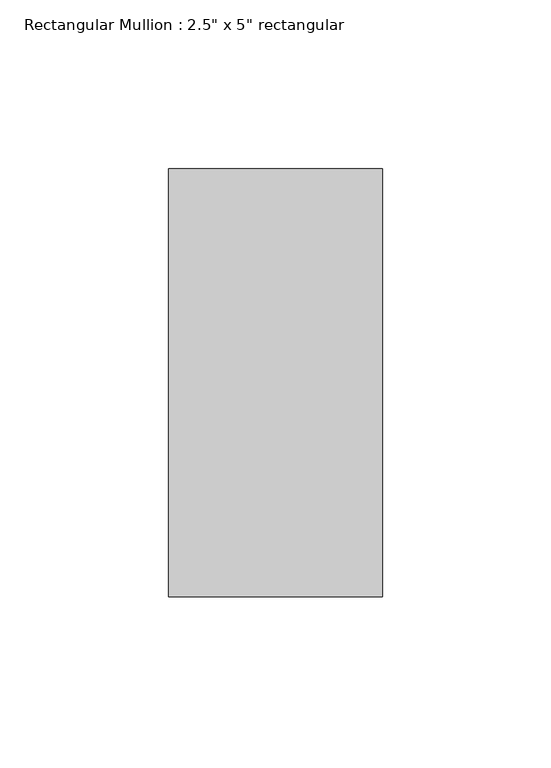
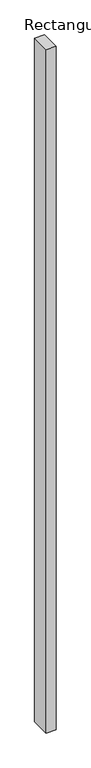
"""IFC4 building model written with IfcOpenShell, lengths in millimetres: member geometry."""

from ifc_helpers import new_model, si_unit, frame, origin, place, context, project, spatial, polyline, outline, extrude, source, transform, mapped, element, save


def member_a33656d8(model_context):
    return source(origin(), model_context, "Body", "SweptSolid", [
        extrude(outline(polyline([(0.0, 63.5), (0.0, -63.5), (-63.5, -63.5), (-63.5, 63.5), (0.0, 63.5)])), frame((0.0, 0.0, -4616.45), z_axis=(0.0, 0.0, 1.0), x_axis=(1.0, 0.0, 0.0)), (0.0, 0.0, 1.0), 4616.45),
    ])


if __name__ == "__main__":
    model = new_model("IFC4")
    model_context = context("Model", 3, world=origin())
    ifc_project = project(units=[si_unit("LENGTHUNIT", "METRE", prefix="MILLI")], contexts=[model_context])
    site = spatial("IfcSite", under=ifc_project)
    building = spatial("IfcBuilding", under=site)
    placement = place(None, origin())
    member_shape = member_a33656d8(model_context)
    element("IfcMember", 1, ObjectType="Rectangular Mullion : 2.5\" x 5\" rectangular", at=placement, inside=building, context=model_context, shape_type="MappedRepresentation", body=[
        mapped(member_shape, transform((0.0, 0.0, 0.0), x_axis=(1.0, 0.0, 0.0), y_axis=(0.0, 1.0, 0.0), z_axis=(0.0, 0.0, 1.0))),
    ])
    save(model, "model.ifc")

# Revit data of these elements
# Type "Rectangular Mullion : 2.5\" x 5\" rectangular"
#   built-in parameter 1007304 = 0.416667 (stored number, unit not read)
#   built-in parameter 1007301 = 0.104167 (stored number, unit not read)
#   built-in parameter 1007300 = 0.104167 (stored number, unit not read)
# Element 1 (IfcMember, "Rectangular Mullion : 2.5\" x 5\" rectangular")
#   Materials on its faces: "Aluminum"
# Materials
#   "Aluminum": class "Metal", colour RGB 247 247 247, transparency 0, Description = "Aluminum 6061", Cost = 0
